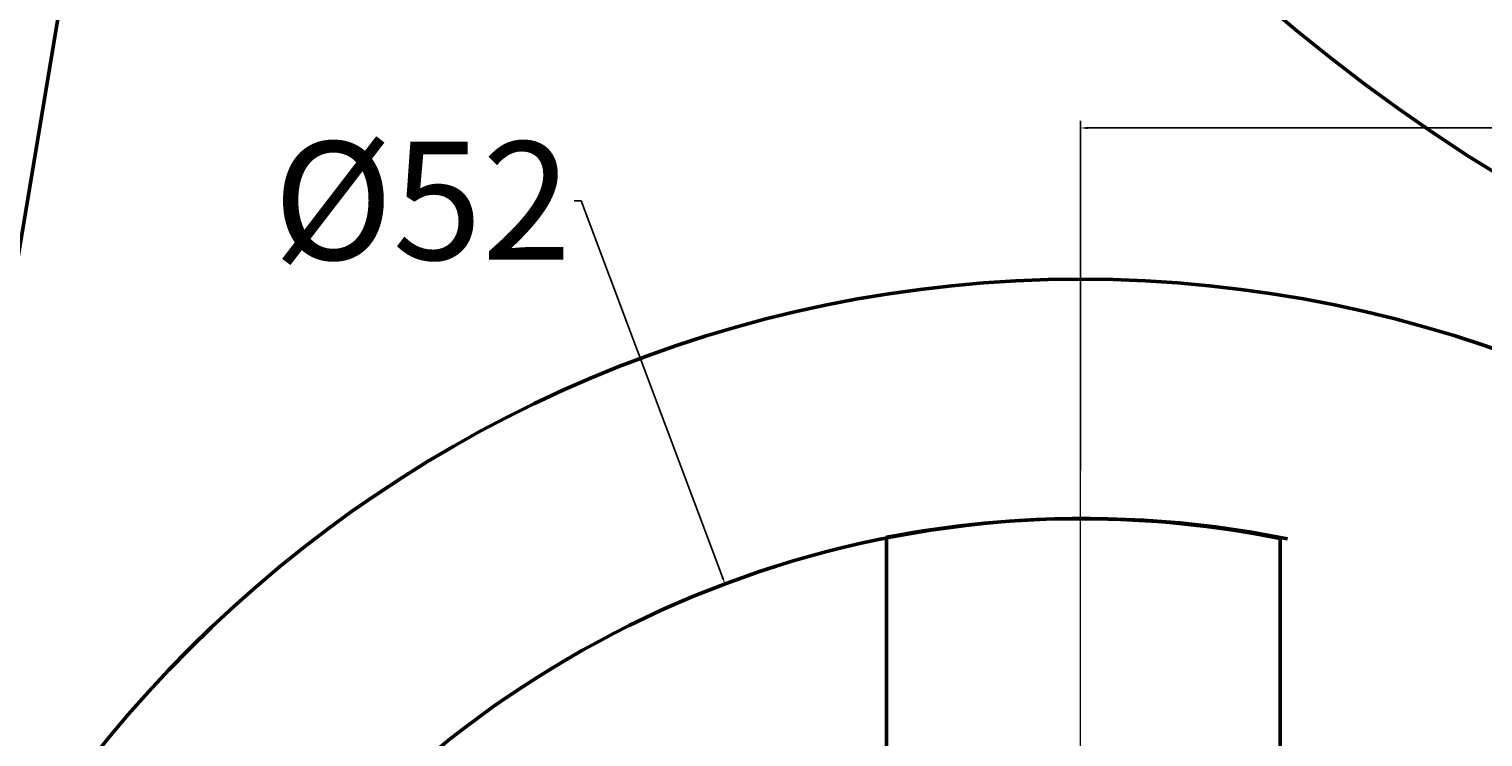
# Model space of a CAD drawing. Units: millimetres. Extents: x -50 to 109, y -46 to 152.
# Tile 4 of 18: x -28 to 9, y 14 to 32. Entities that reach past the tile are written whole.
import ezdxf

# ---------------------------------------------------------------- set-up
doc = ezdxf.new("R2010")
doc.units = ezdxf.units.MM
doc.header["$MEASUREMENT"] = 0
doc.linetypes.add('CENTER', pattern=[50.8, 31.75, -6.35, 6.35, -6.35])
for name, color, linetype, lineweight in [('M-CNTR', 1, 'CENTER', 18), ('M-DIMS', 2, 'Continuous', 25), ('M-OUTL', 7, 'Continuous', 50)]:
    doc.layers.add(name, color=color, linetype=linetype, lineweight=lineweight)
doc.styles.get("Standard").update_dxf_attribs({"font": 'arial.ttf'})
doc.dimstyles.get("Standard").update_dxf_attribs({"dimtxt": 0.18, "dimasz": 0.18, "dimexe": 0.18, "dimexo": 0.0625, "dimgap": 0.09, "dimtad": 0, "dimtih": 1, "dimtoh": 1, "dimdec": 4, "dimzin": 0, "dimdsep": 46, "dimtxsty": 'Standard', "dimcen": 0.09, "dimadec": 0, "dimazin": 0, "dimtfac": 1, "dimtdec": 4, "dimtofl": 0, "dimtmove": 0, "dimatfit": 3, "dimfxl": 1, "dimtolj": 1, "dimtzin": 0, "dimarcsym": 0})

# ---------------------------------------------------------------- blocks, each defined once
blk = doc.blocks.new('*U1')
for p, q in [((-5, 2.851), (-5, -3.294)), ((5, 2.824), (5, -3.323))]:
    blk.add_line(p, q)
blk.add_arc((-0.069, -22.677), 26, 78.7582, 100.9333)
blk = doc.blocks.new('*U2')
at = {"layer": 'M-OUTL', "color": 0, "linetype": 'ByBlock', "lineweight": -2, "transparency": 16777216}
blk.add_blockref('*U1', (-0.855, 15.809), dxfattribs=at)
blk = doc.blocks.new('*U6')
at = {"layer": 'M-CNTR', "color": 0, "transparency": 16777216}
blk.add_line((0, 5.2), (0, 36), dxfattribs=at)
blk = doc.blocks.new('*D19')
at = {"layer": 'Defpoints', "color": 0, "transparency": 16777216}
for p in [(33.152, 29.059), (-0.925, 20.297), (33.152, 19.299)]:
    blk.add_point(p, dxfattribs=at)
at = {"layer": 'M-DIMS', "color": 0, "lineweight": -2, "transparency": 16777216}
for p, q in [((-0.925, 20.359), (-0.925, 29.239)), ((33.152, 19.361), (33.152, 29.239)), ((-0.745, 29.059), (13.882, 29.059)), ((32.972, 29.059), (18.345, 29.059))]:
    blk.add_line(p, q, dxfattribs=at)
at = {"layer": 'M-DIMS', "color": 0, "transparency": 16777216}
for points in [[(-0.745, 29.089), (-0.745, 29.029), (-0.925, 29.059)], [(32.972, 29.089), (32.972, 29.029), (33.152, 29.059)]]:
    blk.add_solid(points, dxfattribs=at)
at = {"layer": 'M-DIMS', "color": 0, "transparency": 16777216, "insert": (16.113, 29.059), "char_height": 0.18, "attachment_point": 5}
blk.add_mtext('\\A1;{\\H16.66667x;34}', dxfattribs=at)
blk = doc.blocks.new('*D24')
at = {"layer": 'Defpoints', "color": 0, "transparency": 16777216}
for p in [(-9.958, 17.477), (8.318, -31.205)]:
    blk.add_point(p, dxfattribs=at)
at = {"layer": 'M-DIMS', "color": 0, "lineweight": -2, "transparency": 16777216}
for p, q in [((-13.793, 27.212), (-13.613, 27.212)), ((-13.613, 27.212), (-10.022, 17.646)), ((-0.91, -6.864), (-0.73, -6.864)), ((-0.82, -6.954), (-0.82, -6.774))]:
    blk.add_line(p, q, dxfattribs=at)
at = {"layer": 'M-DIMS', "color": 0, "transparency": 16777216}
blk.add_solid([(-9.994, 17.656), (-10.05, 17.635), (-9.958, 17.477)], dxfattribs=at)
at = {"layer": 'M-DIMS', "color": 0, "transparency": 16777216, "insert": (-17.649, 27.212), "char_height": 0.18, "attachment_point": 5}
blk.add_mtext('\\A1;{\\H16.66667x;%%C52}', dxfattribs=at)
blk = doc.blocks.new('*D25')
at = {"layer": 'Defpoints', "color": 0, "transparency": 16777216}
for p in [(0.007, 66.376), (-48.373, -6.811), (-0.299, -6.811)]:
    blk.add_point(p, dxfattribs=at)
at = {"layer": 'M-DIMS', "color": 0, "lineweight": -2, "transparency": 16777216}
for p, q in [((-0.056, 66.376), (-48.553, 66.376)), ((-48.373, 66.196), (-48.373, 31.405)), ((-48.373, -6.631), (-48.373, 28.16)), ((-0.361, -6.811), (-48.553, -6.811))]:
    blk.add_line(p, q, dxfattribs=at)
at = {"layer": 'M-DIMS', "color": 0, "transparency": 16777216}
for points in [[(-48.403, 66.196), (-48.343, 66.196), (-48.373, 66.376)], [(-48.403, -6.631), (-48.343, -6.631), (-48.373, -6.811)]]:
    blk.add_solid(points, dxfattribs=at)
at = {"layer": 'M-DIMS', "color": 0, "transparency": 16777216, "insert": (-48.373, 29.782), "char_height": 0.18, "attachment_point": 5}
blk.add_mtext('\\A1;{\\H16.66667x;73}', dxfattribs=at)
blk = doc.blocks.new('*D29')
at = {"layer": 'Defpoints', "color": 0, "transparency": 16777216}
for p in [(21.684, 15.863), (-23.531, -29.431)]:
    blk.add_point(p, dxfattribs=at)
at = {"layer": 'M-DIMS', "color": 0, "lineweight": -2, "transparency": 16777216}
for p, q in [((-1.014, -6.784), (-0.834, -6.784)), ((-0.924, -6.874), (-0.924, -6.694)), ((-37.096, -43.02), (-23.658, -29.559)), ((-37.276, -43.02), (-37.096, -43.02))]:
    blk.add_line(p, q, dxfattribs=at)
at = {"layer": 'M-DIMS', "color": 0, "transparency": 16777216}
blk.add_solid([(-23.68, -29.537), (-23.637, -29.58), (-23.531, -29.431)], dxfattribs=at)
at = {"layer": 'M-DIMS', "color": 0, "transparency": 16777216, "insert": (-37.592, -43.02), "char_height": 0.18, "attachment_point": 5}
blk.add_mtext('\\A1;∅64', dxfattribs=at)

msp = doc.modelspace()

# ---------------------------------------------------------------- linework, layer by layer
at = {"layer": 'M-OUTL'}
msp.add_line((-20.5811, 69.65018), (-32.48503, -1.5038), dxfattribs=at)
msp.add_circle((-0.92366, -6.78396), 32, dxfattribs=at)
for centre, radius, start, end in [((33.197, 66.24997), 45, 180.010473, 359.989527), ((-0.82008, -6.86387), 26, 78.565718, 270.188748)]:
    msp.add_arc(centre, radius, start, end, dxfattribs=at)

# ---------------------------------------------------------------- block references
at = {"layer": 'M-CNTR'}
msp.add_blockref('*U6', (-0.92366, -6.86889), dxfattribs=at)
at = {"layer": 'M-OUTL'}
msp.add_blockref('*U2', (0, 0), dxfattribs=at)

# ---------------------------------------------------------------- dimensions: what is measured, and where the dimension line sits
at = {"layer": 'M-DIMS'}
dim = msp.add_linear_dim(base=(-48.37276, -6.81116), p1=(0.00669, 66.37611), p2=(-0.2986, -6.81116), angle=90, text='{\\H16.66667x;73}', dimstyle='Standard', override={"dimclrd": 0, "dimclre": 0, "dimclrt": 0}, dxfattribs=at)
dim.commit()
dim.dimension.update_dxf_attribs({"geometry": '*D25', "text_midpoint": (-48.37276, 29.78248)})
dim = msp.add_linear_dim(base=(33.15184, 29.05873), p1=(-0.92498, 20.29688), p2=(33.15184, 19.29869), text='{\\H16.66667x;34}', dimstyle='Standard', override={"dimclrd": 0, "dimclre": 0, "dimclrt": 0}, dxfattribs=at)
dim.commit()
dim.dimension.update_dxf_attribs({"geometry": '*D19', "text_midpoint": (16.11343, 29.05873)})
dim = msp.add_diameter_dim_2p(p1=(8.31828, -31.20499), p2=(-9.95844, 17.47726), text='{\\H16.66667x;%%C52}', dimstyle='Standard', override={"dimclrd": 0, "dimclre": 0, "dimclrt": 0}, dxfattribs=at)
dim.commit()
dim.dimension.update_dxf_attribs({"geometry": '*D24', "text_midpoint": (-17.64865, 27.21244), "dimtype": 163})
dim = msp.add_diameter_dim_2p(p1=(21.68387, 15.86332), p2=(-23.53119, -29.43125), dimstyle='Standard', override={"dimdec": 0, "dimlfac": 1, "dimrnd": 0, "dimzin": 0, "dimdsep": 46, "dimlunit": 2}, dxfattribs=at)
dim.commit()
dim.dimension.update_dxf_attribs({"geometry": '*D29', "text_midpoint": (-37.59218, -43.01962), "dimtype": 163})

doc.saveas('drawing.dxf')
